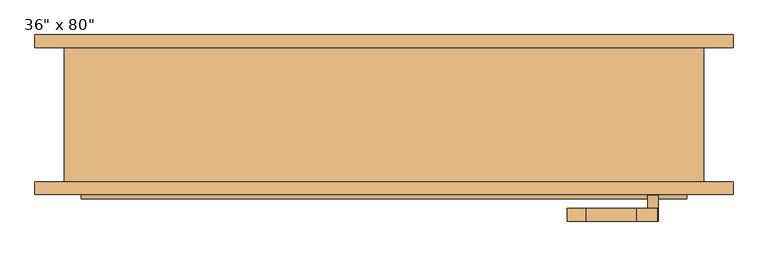
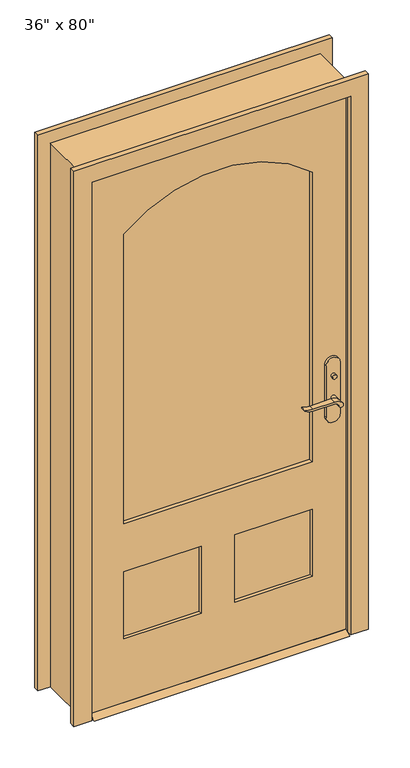
"""IFC4 building model written with IfcOpenShell, lengths in millimetres: door geometry."""

from ifc_helpers import new_model, si_unit, point, frame, frame_2d, origin, place, context, project, spatial, polyline, circle_curve, trimmed, segment, composite_curve, outline, extrude, faceted_brep, source, transform, mapped, element, save


def door_62fd4200(model_context):
    return source(origin(), model_context, "Body", "SolidModel", [
        extrude(outline(polyline([(-63.5, 12.7), (-38.1, 0.0), (-123.825, 0.0), (-98.425, 12.7), (-63.5, 12.7)])), frame((-457.2, 0.0, 0.0), z_axis=(1.0, 0.0, 0.0), x_axis=(0.0, 1.0, 0.0)), (0.0, 0.0, 1.0), 914.4),
        extrude(outline(polyline([(411.4, -43.5), (411.4, -53.5), (401.4, -53.5), (401.4, -43.5), (411.4, -43.5)])), frame((0.0, 0.0, 981.9), z_axis=(0.0, 0.0, 1.0), x_axis=(1.0, 0.0, 0.0)), (0.0, 0.0, 1.0), 30.0),
        extrude(outline(composite_curve([segment(trimmed(circle_curve(frame_2d((996.9, 406.4)), 8.0), [point((996.9, 398.4))], [point((996.9, 414.4))], False, "CARTESIAN"), True, "CONTINUOUS"), segment(trimmed(circle_curve(frame_2d((996.9, 406.4)), 8.0), [point((996.9, 414.4))], [point((996.9, 398.4))], False, "CARTESIAN"), True, "CONTINUOUS")], self_intersect=False)), frame((0.0, -118.425, 0.0), z_axis=(0.0, 1.0, 0.0), x_axis=(0.0, 0.0, 1.0)), (0.0, 0.0, 1.0), 10.0),
        extrude(outline(composite_curve([segment(trimmed(circle_curve(frame_2d((897.1555521, 382.7324871)), 37.2832219), [point((919.0523287, 412.9081363))], [point((934.4, 381.0325667))], False, "CARTESIAN"), True, "CONTINUOUS"), segment(polyline([(934.4, 381.0325667), (934.4, 304.7564091)]), True, "CONTINUOUS"), segment(trimmed(circle_curve(frame_2d((1017.6850638, 304.8227909)), 83.2850902), [point((934.4, 304.7564091))], [point((939.4, 276.4))], True, "CARTESIAN"), True, "CONTINUOUS"), segment(polyline([(939.4, 276.4), (936.6135558, 276.4)]), True, "CONTINUOUS"), segment(trimmed(circle_curve(frame_2d((986.6709207, 308.3396612)), 59.3791355), [point((936.6135558, 276.4))], [point((927.4, 304.7564091))], False, "CARTESIAN"), True, "CONTINUOUS"), segment(polyline([(927.4, 304.7564091), (927.4, 381.0138099)]), True, "CONTINUOUS"), segment(trimmed(circle_curve(frame_2d((909.2738613, 381.0138099)), 18.1261387), [point((927.4, 381.0138099))], [point((914.4, 398.4))], True, "CARTESIAN"), True, "CONTINUOUS"), segment(trimmed(circle_curve(frame_2d((914.4, 406.4)), 8.0), [point((914.4, 398.4))], [point((919.0523287, 412.9081363))], False, "CARTESIAN"), True, "CONTINUOUS")], self_intersect=False)), frame((0.0, -23.5, 0.0), z_axis=(0.0, 1.0, 0.0), x_axis=(0.0, 0.0, 1.0)), (0.0, 0.0, 1.0), 20.0),
        extrude(outline(composite_curve([segment(trimmed(circle_curve(frame_2d((914.4, 406.4)), 8.0), [point((914.3999903, 398.4))], [point((919.0523287, 412.9081363))], False, "CARTESIAN"), True, "CONTINUOUS"), segment(trimmed(circle_curve(frame_2d((897.1555521, 382.7324871)), 37.2832219), [point((919.0523287, 412.9081363))], [point((934.4, 381.0325667))], False, "CARTESIAN"), True, "CONTINUOUS"), segment(polyline([(934.4, 381.0325667), (934.4, 304.7564091)]), True, "CONTINUOUS"), segment(trimmed(circle_curve(frame_2d((1017.6850638, 304.8227909)), 83.2850902), [point((934.4, 304.7564091))], [point((939.4, 276.4))], True, "CARTESIAN"), True, "CONTINUOUS"), segment(polyline([(939.4, 276.4), (936.6135558, 276.4)]), True, "CONTINUOUS"), segment(trimmed(circle_curve(frame_2d((986.6709207, 308.3396612)), 59.3791355), [point((936.6135558, 276.4))], [point((927.4, 304.7564091))], False, "CARTESIAN"), True, "CONTINUOUS"), segment(polyline([(927.4, 304.7564091), (927.4, 381.0138122)]), True, "CONTINUOUS"), segment(trimmed(circle_curve(frame_2d((909.2738682, 381.0138122)), 18.1261318), [point((927.4, 381.0138122))], [point((914.3999903, 398.4))], True, "CARTESIAN"), True, "CONTINUOUS")], self_intersect=False)), frame((0.0, -158.425, 0.0), z_axis=(0.0, 1.0, 0.0), x_axis=(0.0, 0.0, 1.0)), (0.0, 0.0, 1.0), 20.0),
        extrude(outline(composite_curve([segment(trimmed(circle_curve(frame_2d((914.4, 406.4)), 8.0), [point((914.4, 398.4))], [point((914.4, 414.4))], False, "CARTESIAN"), True, "CONTINUOUS"), segment(trimmed(circle_curve(frame_2d((914.4, 406.4)), 8.0), [point((914.4, 414.4))], [point((914.4, 398.4))], False, "CARTESIAN"), True, "CONTINUOUS")], self_intersect=False)), frame((0.0, -53.5, 0.0), z_axis=(0.0, 1.0, 0.0), x_axis=(0.0, 0.0, 1.0)), (0.0, 0.0, 1.0), 30.0),
        extrude(outline(composite_curve([segment(trimmed(circle_curve(frame_2d((914.4, 406.4)), 8.0), [point((914.4, 398.4))], [point((914.4, 414.4))], False, "CARTESIAN"), True, "CONTINUOUS"), segment(trimmed(circle_curve(frame_2d((914.4, 406.4)), 8.0), [point((914.4, 414.4))], [point((914.4, 398.4))], False, "CARTESIAN"), True, "CONTINUOUS")], self_intersect=False)), frame((0.0, -138.425, 0.0), z_axis=(0.0, 1.0, 0.0), x_axis=(0.0, 0.0, 1.0)), (0.0, 0.0, 1.0), 30.0),
        extrude(outline(composite_curve([segment(polyline([(844.4, 431.4), (1039.4, 431.4)]), True, "CONTINUOUS"), segment(trimmed(circle_curve(frame_2d((1039.4, 406.4)), 25.0), [point((1039.4, 431.4))], [point((1039.4, 381.4))], False, "CARTESIAN"), True, "CONTINUOUS"), segment(polyline([(1039.4, 381.4), (844.4, 381.4)]), True, "CONTINUOUS"), segment(trimmed(circle_curve(frame_2d((844.4, 406.4)), 25.0), [point((844.4, 381.4))], [point((844.4, 431.4))], False, "CARTESIAN"), True, "CONTINUOUS")], self_intersect=False)), frame((0.0, -63.5, 0.0), z_axis=(0.0, 1.0, 0.0), x_axis=(0.0, 0.0, 1.0)), (0.0, 0.0, 1.0), 10.0),
        extrude(outline(composite_curve([segment(polyline([(844.4, 431.4), (1039.4, 431.4)]), True, "CONTINUOUS"), segment(trimmed(circle_curve(frame_2d((1039.4, 406.4)), 25.0), [point((1039.4, 431.4))], [point((1039.4, 381.4))], False, "CARTESIAN"), True, "CONTINUOUS"), segment(polyline([(1039.4, 381.4), (844.4, 381.4)]), True, "CONTINUOUS"), segment(trimmed(circle_curve(frame_2d((844.4, 406.4)), 25.0), [point((844.4, 381.4))], [point((844.4, 431.4))], False, "CARTESIAN"), True, "CONTINUOUS")], self_intersect=False)), frame((0.0, -108.425, 0.0), z_axis=(0.0, 1.0, 0.0), x_axis=(0.0, 0.0, 1.0)), (0.0, 0.0, 1.0), 10.0),
        extrude(outline(polyline([(2032.0, -457.2), (12.7, -457.2), (12.7, 457.2), (2032.0, 457.2), (2032.0, -457.2)]), holes=[composite_curve([segment(polyline([(688.975, -336.55), (1784.35, -336.55)]), True, "CONTINUOUS"), segment(trimmed(circle_curve(frame_2d((1401.92125, 0.0)), 509.42875), [point((1784.35, -336.55))], [point((1784.35, 336.55))], True, "CARTESIAN"), True, "CONTINUOUS"), segment(polyline([(1784.35, 336.55), (688.975, 336.55), (688.975, -336.55)]), True, "CONTINUOUS")], self_intersect=False), polyline([(508.0, -60.325), (254.0, -60.325), (254.0, -336.55), (508.0, -336.55), (508.0, -60.325)]), polyline([(508.0, 336.55), (254.0, 336.55), (254.0, 60.325), (508.0, 60.325), (508.0, 336.55)])]), frame((0.0, -98.425, 0.0), z_axis=(0.0, 1.0, 0.0), x_axis=(0.0, 0.0, 1.0)), (0.0, 0.0, 1.0), 34.925),
        faceted_brep([(482.6, -98.425, 0.0), (457.2, -98.425, 0.0), (457.2, -63.5, 0.0), (444.5, -63.5, 0.0), (444.5, -28.575, 0.0), (457.2, -28.575, 0.0), (457.2, 104.775, 0.0), (482.6, 104.775, 0.0), (482.6, 104.775, 2057.4), (482.6, -98.425, 2057.4), (457.2, 104.775, 2032.0), (-457.2, 104.775, 2032.0), (-457.2, 104.775, 0.0), (-482.6, 104.775, 0.0), (-482.6, 104.775, 2057.4), (457.2, -28.575, 2032.0), (444.5, -28.575, 2019.3), (-444.5, -28.575, 2019.3), (-444.5, -28.575, 0.0), (-457.2, -28.575, 0.0), (-457.2, -28.575, 2032.0), (444.5, -63.5, 2019.3), (457.2, -63.5, 2032.0), (-457.2, -63.5, 2032.0), (-457.2, -63.5, 0.0), (-444.5, -63.5, 0.0), (-444.5, -63.5, 2019.3), (457.2, -98.425, 2032.0), (-482.6, -98.425, 2057.4), (-482.6, -98.425, 0.0), (-457.2, -98.425, 0.0), (-457.2, -98.425, 2032.0)], [[[0, 1, 2, 3, 4, 5, 6, 7]], [[7, 8, 9, 0]], [[6, 10, 11, 12, 13, 14, 8, 7]], [[5, 15, 10, 6]], [[4, 16, 17, 18, 19, 20, 15, 5]], [[3, 21, 16, 4]], [[2, 22, 23, 24, 25, 26, 21, 3]], [[1, 27, 22, 2]], [[0, 9, 28, 29, 30, 31, 27, 1]], [[8, 14, 28, 9]], [[15, 20, 11, 10]], [[21, 26, 17, 16]], [[27, 31, 23, 22]], [[29, 13, 12, 19, 18, 25, 24, 30]], [[14, 13, 29, 28]], [[20, 19, 12, 11]], [[26, 25, 18, 17]], [[31, 30, 24, 23]]]),
        extrude(outline(polyline([(-60.325, -75.1416667), (-60.325, -86.7833333), (-336.55, -86.7833333), (-336.55, -75.1416667), (-60.325, -75.1416667)])), frame((0.0, 0.0, 254.0), z_axis=(0.0, 0.0, 1.0), x_axis=(1.0, 0.0, 0.0)), (0.0, 0.0, 1.0), 254.0),
        extrude(outline(polyline([(336.55, -75.1416667), (336.55, -86.7833333), (60.325, -86.7833333), (60.325, -75.1416667), (336.55, -75.1416667)])), frame((0.0, 0.0, 254.0), z_axis=(0.0, 0.0, 1.0), x_axis=(1.0, 0.0, 0.0)), (0.0, 0.0, 1.0), 254.0),
        extrude(outline(composite_curve([segment(polyline([(688.975, -336.55), (688.975, 336.55), (1784.35, 336.55)]), True, "CONTINUOUS"), segment(trimmed(circle_curve(frame_2d((1401.92125, 0.0)), 509.42875), [point((1784.35, 336.55))], [point((1784.35, -336.55))], False, "CARTESIAN"), True, "CONTINUOUS"), segment(polyline([(1784.35, -336.55), (688.975, -336.55)]), True, "CONTINUOUS")], self_intersect=False)), frame((0.0, -84.455, 0.0), z_axis=(0.0, 1.0, 0.0), x_axis=(0.0, 0.0, 1.0)), (0.0, 0.0, 1.0), 6.985),
        extrude(outline(polyline([(0.0, -463.55), (2038.35, -463.55), (2038.35, 463.55), (0.0, 463.55), (0.0, 527.05), (2101.85, 527.05), (2101.85, -527.05), (0.0, -527.05), (0.0, -463.55)])), frame((0.0, 104.775, 0.0), z_axis=(0.0, 1.0, 0.0), x_axis=(0.0, 0.0, 1.0)), (0.0, 0.0, 1.0), 19.05),
        extrude(outline(polyline([(0.0, -463.55), (2038.35, -463.55), (2038.35, 463.55), (0.0, 463.55), (0.0, 527.05), (2101.85, 527.05), (2101.85, -527.05), (0.0, -527.05), (0.0, -463.55)])), frame((0.0, -117.475, 0.0), z_axis=(0.0, 1.0, 0.0), x_axis=(0.0, 0.0, 1.0)), (0.0, 0.0, 1.0), 19.05),
    ])


if __name__ == "__main__":
    model = new_model("IFC4")
    model_context = context("Model", 3, world=origin())
    ifc_project = project(units=[si_unit("LENGTHUNIT", "METRE", prefix="MILLI")], contexts=[model_context])
    site = spatial("IfcSite", under=ifc_project)
    building = spatial("IfcBuilding", under=site)
    placement = place(None, origin())
    door_shape = door_62fd4200(model_context)
    element("IfcDoor", 1, ObjectType="36\" x 80\"", at=placement, inside=building, context=model_context, shape_type="MappedRepresentation", body=[
        mapped(door_shape, transform((0.0, 0.0, 0.0), x_axis=(1.0, 0.0, 0.0), y_axis=(0.0, 1.0, 0.0), z_axis=(0.0, 0.0, 1.0))),
    ])
    save(model, "model.ifc")

# Revit data of these elements
# Type "36\" x 80\""
#   Type Mark = "15"
#   Assembly Code = "B2030100"
#   Analytic Construction = "French door, wood frame with single glass"
#   Threshold Offset [instance default] = 0' - 0 1/2"
#   Thickness = 0' - 1 3/8"
#   Thermal Resistance (R) = 1.0696 (h·ft²·°F)/BTU
#   Swing Angle [instance default] = 90.00°
#   Stiles = 0' - 4 3/4"
#   Rough Width = 3' - 2"
#   Rough Height = 6' - 9"
#   Radius = 1' - 8.05625"
#   Lock Rail = 0' - 7 1/8"
#   Height = 6' - 8"
#   Width = 3' - 0"
#   Heat Transfer Coefficient (U) = 0.9350 BTU/(h·ft²·°F)
#   Door Offset [instance default] = 0' - 0"
#   Bottom Rail = 0' - 9 1/2"
#   Threshold [instance default] = yes
#   Function = 1
#   Exterior Trim [instance default] = yes
#   Trim Material = Cherry
#   Threshold Material = Cherry
#   Panel Material = Cherry
#   Glazing = Glass
#   Frame Material = Cherry
#   Door Handle Material = Aluminum
#   Visual Light Transmittance = 0
#   Solar Heat Gain Coefficient = 0
#   Wall Closure = (empty or 0)
#   Construction Type = (empty or 0)
# Element 1 (IfcDoor, "36\" x 80\"")
#   Materials on its faces: "Cherry", "Aluminum", "Glass"
# Materials
#   "Cherry": class "Wood", colour RGB 226 177 128, transparency 0, Description = "Prunus Serotina", Cost = 0
#   "Glass": class "Glass", colour RGB 0 128 192, transparency 0.75, Description = "Soda Lime Glass", Cost = 0
#   "Aluminum": class "Metal", colour RGB 247 247 247, transparency 0, Description = "Aluminum 6061", Cost = 0
